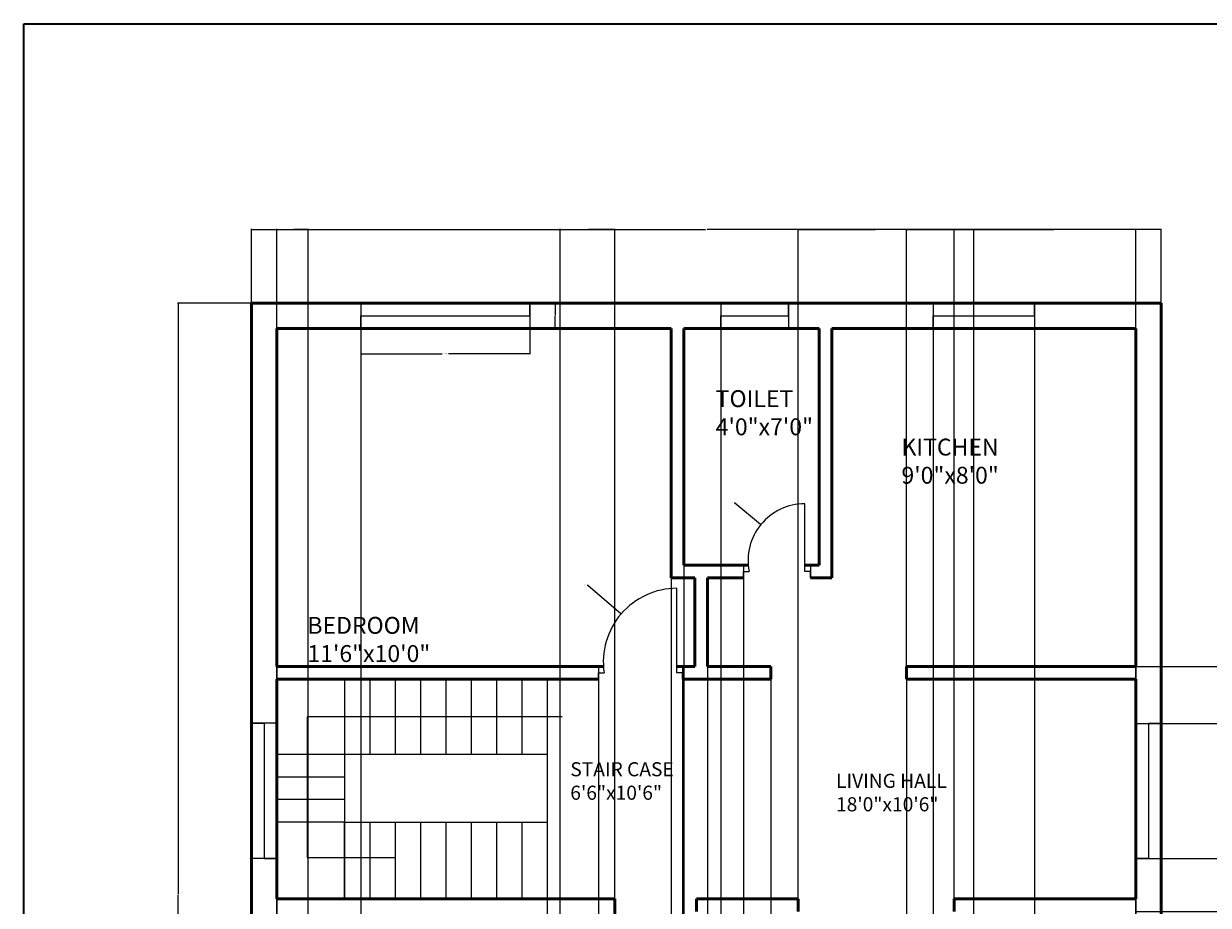
# Model space of a CAD drawing. Units: inches. Extents: x 1860 to 2753, y 1742 to 2419.
# Tile 2 of 4: x 1860 to 2280, y 2106 to 2419. Entities that reach past the tile are written whole.
import ezdxf

# ---------------------------------------------------------------- set-up
doc = ezdxf.new("R2010")
doc.units = ezdxf.units.IN
for name, color, linetype, lineweight in [('A-ANNO-DIMS', 2, 'Continuous', 18), ('A-ANNO-TTLB', 7, 'Continuous', 35), ('A-AREA-IDEN', 7, 'Continuous', 18), ('A-DOOR', 3, 'Continuous', 25), ('A-FLOR-STRS', 7, 'Continuous', 18), ('A-GLAZ', 4, 'Continuous', 18), ('A-WALL', 7, 'Continuous', 50)]:
    doc.layers.add(name, color=color, linetype=linetype, lineweight=lineweight)
doc.styles.get("Standard").update_dxf_attribs({"font": 'arial.ttf'})
doc.dimstyles.get("Standard").update_dxf_attribs({"dimtxt": 0.18, "dimasz": 0.18, "dimexe": 0.18, "dimexo": 0.0625, "dimgap": 0.09, "dimtad": 0, "dimtih": 1, "dimtoh": 1, "dimdec": 4, "dimzin": 0, "dimdsep": 46, "dimtxsty": 'Standard', "dimcen": 0.09, "dimadec": 0, "dimazin": 0, "dimtfac": 1, "dimtdec": 4, "dimtofl": 0, "dimtmove": 0, "dimatfit": 3, "dimfxl": 1, "dimtolj": 1, "dimtzin": 0, "dimarcsym": 0})

# ---------------------------------------------------------------- blocks, each defined once
blk = doc.blocks.new('WIN-24IN')
for p, q in [((0, 9), (0, 0)), ((24, 4.5), (24, 9)), ((24, 9), (24, 0)), ((0, 0), (0, 4.5)), ((0, 4.5), (24, 4.5))]:
    blk.add_line(p, q)
blk = doc.blocks.new('WIN-60IN')
for p, q in [((0, 9), (0, 0)), ((60, 4.5), (60, 9)), ((60, 9), (60, 0)), ((0, 0), (0, 4.5)), ((0, 4.5), (60, 4.5))]:
    blk.add_line(p, q)
blk = doc.blocks.new('*D3')
at = {"layer": 'A-ANNO-DIMS', "color": 0, "lineweight": -2, "transparency": 16777216}
for p, q in [((1979.28, 2311.09), (1979.28, 2301.97)), ((2039.28, 2311.09), (2039.28, 2301.97)), ((1979.46, 2302.15), (2008.16, 2302.15)), ((2039.1, 2302.15), (2010.4, 2302.15))]:
    blk.add_line(p, q, dxfattribs=at)
at = {"layer": 'A-ANNO-DIMS', "color": 0, "transparency": 16777216}
for points in [[(1979.46, 2302.18), (1979.46, 2302.12), (1979.28, 2302.15)], [(2039.1, 2302.18), (2039.1, 2302.12), (2039.28, 2302.15)]]:
    blk.add_solid(points, dxfattribs=at)
at = {"layer": 'Defpoints', "color": 0, "transparency": 16777216}
for p in [(1979.28, 2311.15), (2039.28, 2311.15), (2039.28, 2302.15)]:
    blk.add_point(p, dxfattribs=at)
at = {"layer": 'A-ANNO-DIMS', "color": 0, "transparency": 16777216, "insert": (2009.28, 2302.15), "char_height": 0.18, "attachment_point": 5}
blk.add_mtext('\\A1;WINDOW 60 TYP.', dxfattribs=at)
blk = doc.blocks.new('*D4')
at = {"layer": 'A-ANNO-DIMS', "color": 0, "lineweight": -2, "transparency": 16777216}
for p, q in [((2039.34, 2320.15), (2048.46, 2320.15)), ((2048.28, 2319.97), (2048.28, 2315.83)), ((2048.28, 2311.33), (2048.28, 2315.47)), ((2039.34, 2311.15), (2048.46, 2311.15))]:
    blk.add_line(p, q, dxfattribs=at)
at = {"layer": 'A-ANNO-DIMS', "color": 0, "transparency": 16777216}
for points in [[(2048.25, 2319.97), (2048.31, 2319.97), (2048.28, 2320.15)], [(2048.25, 2311.33), (2048.31, 2311.33), (2048.28, 2311.15)]]:
    blk.add_solid(points, dxfattribs=at)
at = {"layer": 'Defpoints', "color": 0, "transparency": 16777216}
for p in [(2039.28, 2320.15), (2048.28, 2320.15), (2039.28, 2311.15)]:
    blk.add_point(p, dxfattribs=at)
at = {"layer": 'A-ANNO-DIMS', "color": 0, "transparency": 16777216, "insert": (2048.28, 2315.65), "char_height": 0.18, "attachment_point": 5}
blk.add_mtext('\\A1;9 TYP.', dxfattribs=at)
blk = doc.blocks.new('*D7')
at = {"layer": 'A-ANNO-DIMS', "color": 0, "lineweight": -2, "transparency": 16777216}
for p, q in [((1940.47, 2320.21), (1940.47, 2346.43)), ((1940.65, 2346.25), (2101.68, 2346.25)), ((2263.29, 2346.25), (2102.26, 2346.25)), ((2263.47, 2320.21), (2263.47, 2346.43))]:
    blk.add_line(p, q, dxfattribs=at)
at = {"layer": 'A-ANNO-DIMS', "color": 0, "transparency": 16777216}
for points in [[(1940.65, 2346.28), (1940.65, 2346.22), (1940.47, 2346.25)], [(2263.29, 2346.28), (2263.29, 2346.22), (2263.47, 2346.25)]]:
    blk.add_solid(points, dxfattribs=at)
at = {"layer": 'Defpoints', "color": 0, "transparency": 16777216}
for p in [(2263.47, 2346.25), (1940.47, 2320.15), (2263.47, 2320.15)]:
    blk.add_point(p, dxfattribs=at)
at = {"layer": 'A-ANNO-DIMS', "color": 0, "transparency": 16777216, "insert": (2101.97, 2346.25), "char_height": 0.18, "attachment_point": 5}
blk.add_mtext('\\A1;323', dxfattribs=at)
blk = doc.blocks.new('*D8')
at = {"layer": 'A-ANNO-DIMS', "color": 0, "lineweight": -2, "transparency": 16777216}
for p, q in [((1940.41, 2320.15), (1914.19, 2320.15)), ((1914.37, 2319.97), (1914.37, 2110.33)), ((1914.37, 1900.33), (1914.37, 2109.97)), ((1940.41, 1900.15), (1914.19, 1900.15))]:
    blk.add_line(p, q, dxfattribs=at)
at = {"layer": 'A-ANNO-DIMS', "color": 0, "transparency": 16777216}
for points in [[(1914.34, 2319.97), (1914.4, 2319.97), (1914.37, 2320.15)], [(1914.34, 1900.33), (1914.4, 1900.33), (1914.37, 1900.15)]]:
    blk.add_solid(points, dxfattribs=at)
at = {"layer": 'Defpoints', "color": 0, "transparency": 16777216}
for p in [(1914.37, 2320.15), (1940.47, 2320.15), (1940.47, 1900.15)]:
    blk.add_point(p, dxfattribs=at)
at = {"layer": 'A-ANNO-DIMS', "color": 0, "transparency": 16777216, "insert": (1914.37, 2110.15), "char_height": 0.18, "attachment_point": 5}
blk.add_mtext('\\A1;420', dxfattribs=at)
blk = doc.blocks.new('*D9')
at = {"layer": 'A-ANNO-DIMS', "color": 0, "lineweight": -2, "transparency": 16777216}
for p, q in [((1949.47, 2311.09), (1949.47, 1873.87)), ((1979.28, 2311.09), (1979.28, 1873.87)), ((1949.65, 1874.05), (1964, 1874.05)), ((1979.1, 1874.05), (1964.75, 1874.05))]:
    blk.add_line(p, q, dxfattribs=at)
at = {"layer": 'A-ANNO-DIMS', "color": 0, "transparency": 16777216}
for points in [[(1949.65, 1874.08), (1949.65, 1874.02), (1949.47, 1874.05)], [(1979.1, 1874.08), (1979.1, 1874.02), (1979.28, 1874.05)]]:
    blk.add_solid(points, dxfattribs=at)
at = {"layer": 'Defpoints', "color": 0, "transparency": 16777216}
for p in [(1949.47, 2311.15), (1979.28, 2311.15), (1979.28, 1874.05)]:
    blk.add_point(p, dxfattribs=at)
at = {"layer": 'A-ANNO-DIMS', "color": 0, "transparency": 16777216, "insert": (1964.37, 1874.05), "char_height": 0.18, "attachment_point": 5}
blk.add_mtext('\\A1;29.81', dxfattribs=at)
blk = doc.blocks.new('*D10')
at = {"layer": 'A-ANNO-DIMS', "color": 0, "lineweight": -2, "transparency": 16777216}
for p, q in [((2093.97, 2311.09), (2093.97, 1873.87)), ((2107.08, 2311.09), (2107.08, 1873.87)), ((2094.15, 1874.05), (2100.07, 1874.05)), ((2106.9, 1874.05), (2100.98, 1874.05))]:
    blk.add_line(p, q, dxfattribs=at)
at = {"layer": 'A-ANNO-DIMS', "color": 0, "transparency": 16777216}
for points in [[(2094.15, 1874.08), (2094.15, 1874.02), (2093.97, 1874.05)], [(2106.9, 1874.08), (2106.9, 1874.02), (2107.08, 1874.05)]]:
    blk.add_solid(points, dxfattribs=at)
at = {"layer": 'Defpoints', "color": 0, "transparency": 16777216}
for p in [(2093.97, 2311.15), (2107.08, 2311.15), (2107.08, 1874.05)]:
    blk.add_point(p, dxfattribs=at)
at = {"layer": 'A-ANNO-DIMS', "color": 0, "transparency": 16777216, "insert": (2100.52, 1874.05), "char_height": 0.18, "attachment_point": 5}
blk.add_mtext('\\A1;13.107', dxfattribs=at)
blk = doc.blocks.new('*D11')
at = {"layer": 'A-ANNO-DIMS', "color": 0, "lineweight": -2, "transparency": 16777216}
for p, q in [((2182.45, 2311.09), (2182.45, 1873.87)), ((2218.45, 2311.09), (2218.45, 1873.87)), ((2182.63, 1874.05), (2200.24, 1874.05)), ((2218.27, 1874.05), (2200.67, 1874.05))]:
    blk.add_line(p, q, dxfattribs=at)
at = {"layer": 'A-ANNO-DIMS', "color": 0, "transparency": 16777216}
for points in [[(2182.63, 1874.08), (2182.63, 1874.02), (2182.45, 1874.05)], [(2218.27, 1874.08), (2218.27, 1874.02), (2218.45, 1874.05)]]:
    blk.add_solid(points, dxfattribs=at)
at = {"layer": 'Defpoints', "color": 0, "transparency": 16777216}
for p in [(2182.45, 2311.15), (2218.45, 2311.15), (2218.45, 1874.05)]:
    blk.add_point(p, dxfattribs=at)
at = {"layer": 'A-ANNO-DIMS', "color": 0, "transparency": 16777216, "insert": (2200.45, 1874.05), "char_height": 0.18, "attachment_point": 5}
blk.add_mtext('\\A1;36', dxfattribs=at)
blk = doc.blocks.new('*D12')
at = {"layer": 'A-ANNO-DIMS', "color": 0, "lineweight": -2, "transparency": 16777216}
for p, q in [((2218.45, 2311.09), (2218.45, 1873.87)), ((2254.47, 2311.09), (2254.47, 1873.87)), ((2218.63, 1874.05), (2236, 1874.05)), ((2254.29, 1874.05), (2236.93, 1874.05))]:
    blk.add_line(p, q, dxfattribs=at)
at = {"layer": 'A-ANNO-DIMS', "color": 0, "transparency": 16777216}
for points in [[(2218.63, 1874.08), (2218.63, 1874.02), (2218.45, 1874.05)], [(2254.29, 1874.08), (2254.29, 1874.02), (2254.47, 1874.05)]]:
    blk.add_solid(points, dxfattribs=at)
at = {"layer": 'Defpoints', "color": 0, "transparency": 16777216}
for p in [(2218.45, 2311.15), (2254.47, 2311.15), (2254.47, 1874.05)]:
    blk.add_point(p, dxfattribs=at)
at = {"layer": 'A-ANNO-DIMS', "color": 0, "transparency": 16777216, "insert": (2236.46, 1874.05), "char_height": 0.18, "attachment_point": 5}
blk.add_mtext('\\A1;36.016', dxfattribs=at)
blk = doc.blocks.new('*D13')
at = {"layer": 'A-ANNO-DIMS', "color": 0, "lineweight": -2, "transparency": 16777216}
for p, q in [((1949.47, 1909.21), (1949.47, 2346.43)), ((1949.65, 2346.25), (1954.55, 2346.25)), ((1960.35, 2346.25), (1955.46, 2346.25)), ((1960.53, 1909.21), (1960.53, 2346.43))]:
    blk.add_line(p, q, dxfattribs=at)
at = {"layer": 'A-ANNO-DIMS', "color": 0, "transparency": 16777216}
for points in [[(1949.65, 2346.28), (1949.65, 2346.22), (1949.47, 2346.25)], [(1960.35, 2346.28), (1960.35, 2346.22), (1960.53, 2346.25)]]:
    blk.add_solid(points, dxfattribs=at)
at = {"layer": 'Defpoints', "color": 0, "transparency": 16777216}
for p in [(1960.53, 2346.25), (1949.47, 1909.15), (1960.53, 1909.15)]:
    blk.add_point(p, dxfattribs=at)
at = {"layer": 'A-ANNO-DIMS', "color": 0, "transparency": 16777216, "insert": (1955, 2346.25), "char_height": 0.18, "attachment_point": 5}
blk.add_mtext('\\A1;11.063', dxfattribs=at)
blk = doc.blocks.new('*D15')
at = {"layer": 'A-ANNO-DIMS', "color": 0, "lineweight": -2, "transparency": 16777216}
for p, q in [((2050.02, 1909.21), (2050.02, 2346.43)), ((2050.2, 2346.25), (2059.36, 2346.25)), ((2069.29, 2346.25), (2060.13, 2346.25)), ((2069.47, 1920.76), (2069.47, 2346.43))]:
    blk.add_line(p, q, dxfattribs=at)
at = {"layer": 'A-ANNO-DIMS', "color": 0, "transparency": 16777216}
for points in [[(2050.2, 2346.28), (2050.2, 2346.22), (2050.02, 2346.25)], [(2069.29, 2346.28), (2069.29, 2346.22), (2069.47, 2346.25)]]:
    blk.add_solid(points, dxfattribs=at)
at = {"layer": 'Defpoints', "color": 0, "transparency": 16777216}
for p in [(2069.47, 2346.25), (2069.47, 1920.7), (2050.02, 1909.15)]:
    blk.add_point(p, dxfattribs=at)
at = {"layer": 'A-ANNO-DIMS', "color": 0, "transparency": 16777216, "insert": (2059.74, 2346.25), "char_height": 0.18, "attachment_point": 5}
blk.add_mtext('\\A1;19.45', dxfattribs=at)
blk = doc.blocks.new('*D19')
at = {"layer": 'A-ANNO-DIMS', "color": 0, "lineweight": -2, "transparency": 16777216}
for p, q in [((2263.53, 2122.97), (2289.75, 2122.97)), ((2289.57, 2122.79), (2289.57, 2113.74)), ((2289.57, 2104.33), (2289.57, 2113.38)), ((2254.53, 2104.15), (2289.75, 2104.15))]:
    blk.add_line(p, q, dxfattribs=at)
at = {"layer": 'A-ANNO-DIMS', "color": 0, "transparency": 16777216}
for points in [[(2289.54, 2122.79), (2289.6, 2122.79), (2289.57, 2122.97)], [(2289.54, 2104.33), (2289.6, 2104.33), (2289.57, 2104.15)]]:
    blk.add_solid(points, dxfattribs=at)
at = {"layer": 'Defpoints', "color": 0, "transparency": 16777216}
for p in [(2263.47, 2122.97), (2289.57, 2122.97), (2254.47, 2104.15)]:
    blk.add_point(p, dxfattribs=at)
at = {"layer": 'A-ANNO-DIMS', "color": 0, "transparency": 16777216, "insert": (2289.57, 2113.56), "char_height": 0.18, "attachment_point": 5}
blk.add_mtext('\\A1;18.82', dxfattribs=at)
blk = doc.blocks.new('*D20')
at = {"layer": 'A-ANNO-DIMS', "color": 0, "lineweight": -2, "transparency": 16777216}
for p, q in [((2263.53, 2170.97), (2289.75, 2170.97)), ((2289.57, 2170.79), (2289.57, 2147.15)), ((2289.57, 2123.15), (2289.57, 2146.79)), ((2263.53, 2122.97), (2289.75, 2122.97))]:
    blk.add_line(p, q, dxfattribs=at)
at = {"layer": 'A-ANNO-DIMS', "color": 0, "transparency": 16777216}
for points in [[(2289.54, 2170.79), (2289.6, 2170.79), (2289.57, 2170.97)], [(2289.54, 2123.15), (2289.6, 2123.15), (2289.57, 2122.97)]]:
    blk.add_solid(points, dxfattribs=at)
at = {"layer": 'Defpoints', "color": 0, "transparency": 16777216}
for p in [(2263.47, 2170.97), (2289.57, 2170.97), (2263.47, 2122.97)]:
    blk.add_point(p, dxfattribs=at)
at = {"layer": 'A-ANNO-DIMS', "color": 0, "transparency": 16777216, "insert": (2289.57, 2146.97), "char_height": 0.18, "attachment_point": 5}
blk.add_mtext('\\A1;48', dxfattribs=at)
blk = doc.blocks.new('*D21')
at = {"layer": 'A-ANNO-DIMS', "color": 0, "lineweight": -2, "transparency": 16777216}
for p, q in [((2254.53, 2191.15), (2289.75, 2191.15)), ((2289.57, 2190.97), (2289.57, 2181.24)), ((2289.57, 2171.15), (2289.57, 2180.88)), ((2263.53, 2170.97), (2289.75, 2170.97))]:
    blk.add_line(p, q, dxfattribs=at)
at = {"layer": 'A-ANNO-DIMS', "color": 0, "transparency": 16777216}
for points in [[(2289.54, 2190.97), (2289.6, 2190.97), (2289.57, 2191.15)], [(2289.54, 2171.15), (2289.6, 2171.15), (2289.57, 2170.97)]]:
    blk.add_solid(points, dxfattribs=at)
at = {"layer": 'Defpoints', "color": 0, "transparency": 16777216}
for p in [(2254.47, 2191.15), (2289.57, 2191.15), (2263.47, 2170.97)]:
    blk.add_point(p, dxfattribs=at)
at = {"layer": 'A-ANNO-DIMS', "color": 0, "transparency": 16777216, "insert": (2289.57, 2181.06), "char_height": 0.18, "attachment_point": 5}
blk.add_mtext('\\A1;20.18', dxfattribs=at)
blk = doc.blocks.new('*D22')
at = {"layer": 'A-ANNO-DIMS', "color": 0, "lineweight": -2, "transparency": 16777216}
for p, q in [((2196.96, 1972.21), (2196.96, 2346.43)), ((2197.14, 2346.25), (2225.34, 2346.25)), ((2254.29, 2346.25), (2226.09, 2346.25)), ((2254.47, 1972.21), (2254.47, 2346.43))]:
    blk.add_line(p, q, dxfattribs=at)
at = {"layer": 'A-ANNO-DIMS', "color": 0, "transparency": 16777216}
for points in [[(2197.14, 2346.28), (2197.14, 2346.22), (2196.96, 2346.25)], [(2254.29, 2346.28), (2254.29, 2346.22), (2254.47, 2346.25)]]:
    blk.add_solid(points, dxfattribs=at)
at = {"layer": 'Defpoints', "color": 0, "transparency": 16777216}
for p in [(2254.47, 2346.25), (2196.96, 1972.15), (2254.47, 1972.15)]:
    blk.add_point(p, dxfattribs=at)
at = {"layer": 'A-ANNO-DIMS', "color": 0, "transparency": 16777216, "insert": (2225.71, 2346.25), "char_height": 0.18, "attachment_point": 5}
blk.add_mtext('\\A1;57.51', dxfattribs=at)
blk = doc.blocks.new('*D24')
at = {"layer": 'A-ANNO-DIMS', "color": 0, "lineweight": -2, "transparency": 16777216}
for p, q in [((2134.51, 2108.71), (2134.51, 2346.43)), ((2134.69, 2346.25), (2161.84, 2346.25)), ((2189.78, 2346.25), (2162.63, 2346.25)), ((2189.96, 2108.71), (2189.96, 2346.43))]:
    blk.add_line(p, q, dxfattribs=at)
at = {"layer": 'A-ANNO-DIMS', "color": 0, "transparency": 16777216}
for points in [[(2134.69, 2346.28), (2134.69, 2346.22), (2134.51, 2346.25)], [(2189.78, 2346.28), (2189.78, 2346.22), (2189.96, 2346.25)]]:
    blk.add_solid(points, dxfattribs=at)
at = {"layer": 'Defpoints', "color": 0, "transparency": 16777216}
for p in [(2189.96, 2346.25), (2134.51, 2108.65), (2189.96, 2108.65)]:
    blk.add_point(p, dxfattribs=at)
at = {"layer": 'A-ANNO-DIMS', "color": 0, "transparency": 16777216, "insert": (2162.24, 2346.25), "char_height": 0.18, "attachment_point": 5}
blk.add_mtext('\\A1;55.45', dxfattribs=at)
blk = doc.blocks.new('*D25')
at = {"layer": 'A-ANNO-DIMS', "color": 0, "lineweight": -2, "transparency": 16777216}
for p, q in [((2124.88, 2186.59), (2124.88, 1873.87)), ((2172.98, 2186.59), (2172.98, 1873.87)), ((2125.06, 1874.05), (2148.62, 1874.05)), ((2172.8, 1874.05), (2149.24, 1874.05))]:
    blk.add_line(p, q, dxfattribs=at)
at = {"layer": 'A-ANNO-DIMS', "color": 0, "transparency": 16777216}
for points in [[(2125.06, 1874.08), (2125.06, 1874.02), (2124.88, 1874.05)], [(2172.8, 1874.08), (2172.8, 1874.02), (2172.98, 1874.05)]]:
    blk.add_solid(points, dxfattribs=at)
at = {"layer": 'Defpoints', "color": 0, "transparency": 16777216}
for p in [(2124.88, 2186.65), (2172.98, 2186.65), (2172.98, 1874.05)]:
    blk.add_point(p, dxfattribs=at)
at = {"layer": 'A-ANNO-DIMS', "color": 0, "transparency": 16777216, "insert": (2148.93, 1874.05), "char_height": 0.18, "attachment_point": 5}
blk.add_mtext('\\A1;48.1', dxfattribs=at)
blk = doc.blocks.new('*D26')
at = {"layer": 'A-ANNO-DIMS', "color": 0, "lineweight": -2, "transparency": 16777216}
for p, q in [((2172.98, 2191.21), (2172.98, 2346.43)), ((2173.16, 2346.25), (2213.33, 2346.25)), ((2254.29, 2346.25), (2214.12, 2346.25)), ((2254.47, 2191.21), (2254.47, 2346.43))]:
    blk.add_line(p, q, dxfattribs=at)
at = {"layer": 'A-ANNO-DIMS', "color": 0, "transparency": 16777216}
for points in [[(2173.16, 2346.28), (2173.16, 2346.22), (2172.98, 2346.25)], [(2254.29, 2346.28), (2254.29, 2346.22), (2254.47, 2346.25)]]:
    blk.add_solid(points, dxfattribs=at)
at = {"layer": 'Defpoints', "color": 0, "transparency": 16777216}
for p in [(2254.47, 2346.25), (2172.98, 2191.15), (2254.47, 2191.15)]:
    blk.add_point(p, dxfattribs=at)
at = {"layer": 'A-ANNO-DIMS', "color": 0, "transparency": 16777216, "insert": (2213.73, 2346.25), "char_height": 0.18, "attachment_point": 5}
blk.add_mtext('\\A1;81.49', dxfattribs=at)
blk = doc.blocks.new('*D27')
at = {"layer": 'A-ANNO-DIMS', "color": 0, "lineweight": -2, "transparency": 16777216}
for p, q in [((2089.47, 2311.09), (2089.47, 1873.87)), ((2093.97, 2311.09), (2093.97, 1873.87)), ((2089.65, 1874.05), (2091.46, 1874.05)), ((2093.79, 1874.05), (2091.98, 1874.05))]:
    blk.add_line(p, q, dxfattribs=at)
at = {"layer": 'A-ANNO-DIMS', "color": 0, "transparency": 16777216}
for points in [[(2089.65, 1874.08), (2089.65, 1874.02), (2089.47, 1874.05)], [(2093.79, 1874.08), (2093.79, 1874.02), (2093.97, 1874.05)]]:
    blk.add_solid(points, dxfattribs=at)
at = {"layer": 'Defpoints', "color": 0, "transparency": 16777216}
for p in [(2089.47, 2311.15), (2093.97, 2311.15), (2093.97, 1874.05)]:
    blk.add_point(p, dxfattribs=at)
at = {"layer": 'A-ANNO-DIMS', "color": 0, "transparency": 16777216, "insert": (2091.72, 1874.05), "char_height": 0.18, "attachment_point": 5}
blk.add_mtext('\\A1;4.5', dxfattribs=at)
blk = doc.blocks.new('*D28')
at = {"layer": 'A-ANNO-DIMS', "color": 0, "lineweight": -2, "transparency": 16777216}
for p, q in [((2102.3, 2222.59), (2102.3, 1873.87)), ((2115.14, 2222.59), (2115.14, 1873.87)), ((2102.48, 1874.05), (2108.27, 1874.05)), ((2114.96, 1874.05), (2109.18, 1874.05))]:
    blk.add_line(p, q, dxfattribs=at)
at = {"layer": 'A-ANNO-DIMS', "color": 0, "transparency": 16777216}
for points in [[(2102.48, 1874.08), (2102.48, 1874.02), (2102.3, 1874.05)], [(2114.96, 1874.08), (2114.96, 1874.02), (2115.14, 1874.05)]]:
    blk.add_solid(points, dxfattribs=at)
at = {"layer": 'Defpoints', "color": 0, "transparency": 16777216}
for p in [(2102.3, 2222.65), (2115.14, 2222.65), (2115.14, 1874.05)]:
    blk.add_point(p, dxfattribs=at)
at = {"layer": 'A-ANNO-DIMS', "color": 0, "transparency": 16777216, "insert": (2108.72, 1874.05), "char_height": 0.18, "attachment_point": 5}
blk.add_mtext('\\A1;12.834', dxfattribs=at)
blk = doc.blocks.new('*D29')
at = {"layer": 'A-ANNO-DIMS', "color": 0, "lineweight": -2, "transparency": 16777216}
for p, q in [((2102.3, 2191.09), (2102.3, 1873.87)), ((2093.49, 2186.59), (2093.49, 1873.87)), ((2093.67, 1874.05), (2097.51, 1874.05)), ((2102.12, 1874.05), (2098.29, 1874.05))]:
    blk.add_line(p, q, dxfattribs=at)
at = {"layer": 'A-ANNO-DIMS', "color": 0, "transparency": 16777216}
for points in [[(2093.67, 1874.08), (2093.67, 1874.02), (2093.49, 1874.05)], [(2102.12, 1874.08), (2102.12, 1874.02), (2102.3, 1874.05)]]:
    blk.add_solid(points, dxfattribs=at)
at = {"layer": 'Defpoints', "color": 0, "transparency": 16777216}
for p in [(2102.3, 2191.15), (2093.49, 2186.65), (2102.3, 1874.05)]:
    blk.add_point(p, dxfattribs=at)
at = {"layer": 'A-ANNO-DIMS', "color": 0, "transparency": 16777216, "insert": (2097.9, 1874.05), "char_height": 0.18, "attachment_point": 5}
blk.add_mtext('\\A1;8.809', dxfattribs=at)
blk = doc.blocks.new('*D30')
at = {"layer": 'A-ANNO-DIMS', "color": 0, "lineweight": -2, "transparency": 16777216}
for p, q in [((2045.47, 2186.59), (2045.47, 1873.87)), ((2063.65, 2186.59), (2063.65, 1873.87)), ((2045.65, 1874.05), (2054.11, 1874.05)), ((2063.47, 1874.05), (2055.02, 1874.05))]:
    blk.add_line(p, q, dxfattribs=at)
at = {"layer": 'A-ANNO-DIMS', "color": 0, "transparency": 16777216}
for points in [[(2045.65, 1874.08), (2045.65, 1874.02), (2045.47, 1874.05)], [(2063.47, 1874.08), (2063.47, 1874.02), (2063.65, 1874.05)]]:
    blk.add_solid(points, dxfattribs=at)
at = {"layer": 'Defpoints', "color": 0, "transparency": 16777216}
for p in [(2045.47, 2186.65), (2063.65, 2186.65), (2063.65, 1874.05)]:
    blk.add_point(p, dxfattribs=at)
at = {"layer": 'A-ANNO-DIMS', "color": 0, "transparency": 16777216, "insert": (2054.56, 1874.05), "char_height": 0.18, "attachment_point": 5}
blk.add_mtext('\\A1;18.183', dxfattribs=at)
blk = doc.blocks.new('*D53')
at = {"layer": 'A-ANNO-DIMS', "color": 0, "lineweight": -2, "transparency": 16777216}
for p, q in [((2059.64, 2220.05), (2059.82, 2220.05)), ((2059.82, 2220.05), (2071.56, 2209.94)), ((2091.4, 2192.77), (2091.58, 2192.77)), ((2091.49, 2192.68), (2091.49, 2192.86))]:
    blk.add_line(p, q, dxfattribs=at)
at = {"layer": 'A-ANNO-DIMS', "color": 0, "transparency": 16777216}
blk.add_solid([(2071.58, 2209.96), (2071.54, 2209.92), (2071.7, 2209.82)], dxfattribs=at)
at = {"layer": 'Defpoints', "color": 0, "transparency": 16777216}
for p in [(2071.7, 2209.82), (2091.49, 2192.77)]:
    blk.add_point(p, dxfattribs=at)
at = {"layer": 'A-ANNO-DIMS', "color": 0, "transparency": 16777216, "insert": (2059.16, 2220.05), "char_height": 0.18, "attachment_point": 5}
blk.add_mtext('\\A1;R26.13', dxfattribs=at)
blk = doc.blocks.new('*D55')
at = {"layer": 'A-ANNO-DIMS', "color": 0, "lineweight": -2, "transparency": 16777216}
for p, q in [((2111.84, 2249.23), (2112.02, 2249.23)), ((2112.02, 2249.23), (2121.21, 2241.67)), ((2136.79, 2228.77), (2136.97, 2228.77)), ((2136.88, 2228.68), (2136.88, 2228.86))]:
    blk.add_line(p, q, dxfattribs=at)
at = {"layer": 'A-ANNO-DIMS', "color": 0, "transparency": 16777216}
blk.add_solid([(2121.22, 2241.7), (2121.19, 2241.65), (2121.34, 2241.56)], dxfattribs=at)
at = {"layer": 'Defpoints', "color": 0, "transparency": 16777216}
for p in [(2121.34, 2241.56), (2136.88, 2228.77)]:
    blk.add_point(p, dxfattribs=at)
at = {"layer": 'A-ANNO-DIMS', "color": 0, "transparency": 16777216, "insert": (2111.29, 2249.23), "char_height": 0.18, "attachment_point": 5}
blk.add_mtext('\\A1;R20.123', dxfattribs=at)

msp = doc.modelspace()

# ---------------------------------------------------------------- linework, layer by layer
at = {"layer": 'A-ANNO-TTLB'}
msp.add_lwpolyline([(1859.5561, 2419.29), (2753.3204, 2419.29), (2753.3204, 1741.6035), (1859.5561, 1741.6035)], close=True, dxfattribs=at)
at = {"layer": 'A-DOOR'}
for p, q in [((2136.8843, 2224.8976), (2136.8843, 2248.8976)), ((2115.1377, 2227.1476), (2115.1377, 2222.6476)), ((2138.8843, 2227.1476), (2138.8843, 2222.6476)), ((2115.1377, 2222.6476), (2115.1377, 2224.8976)), ((2115.1377, 2224.8976), (2117.1377, 2224.8976)), ((2138.8843, 2224.8976), (2136.8843, 2224.8976)), ((2138.8843, 2222.6476), (2138.8843, 2224.8976)), ((2091.4949, 2188.8976), (2091.4949, 2218.8976)), ((2063.6532, 2191.1476), (2063.6532, 2191.1476)), ((2063.6532, 2191.1476), (2063.6532, 2186.6476)), ((2063.6532, 2186.6476), (2063.6532, 2188.8976)), ((2063.6532, 2188.8976), (2065.6532, 2188.8976)), ((2093.4949, 2188.8976), (2091.4949, 2188.8976)), ((2093.4949, 2191.1476), (2093.4949, 2186.6476)), ((2093.4949, 2186.6476), (2093.4949, 2188.8976))]:
    msp.add_line(p, q, dxfattribs=at)
for centre, radius, end in [((2136.8843, 2228.7741), 20.1235, 191.10666), ((2091.4949, 2192.7677), 26.1299, 188.517535)]:
    msp.add_arc(centre, radius, 90, end, dxfattribs=at)
at = {"layer": 'A-FLOR-STRS'}
for p, q in [((1949.4703, 2186.6476), (1973.4703, 2186.6476)), ((1973.4703, 2186.6476), (1973.4703, 2108.6476)), ((1982.4703, 2186.6476), (1982.4703, 2159.9296)), ((1991.4703, 2186.6476), (1991.4703, 2159.9296)), ((2000.4703, 2186.6476), (2000.4703, 2159.9296)), ((2009.4703, 2186.6476), (2009.4703, 2159.9296)), ((2018.4703, 2186.6476), (2018.4703, 2159.9296)), ((2027.4703, 2186.6476), (2027.4703, 2159.9296)), ((2036.4703, 2186.6476), (2036.4703, 2159.9296)), ((2045.4703, 2186.6476), (2045.4703, 2159.9296)), ((2050.7657, 2173.2886), (1960.21, 2173.2886)), ((1960.21, 2173.2886), (1960.21, 2123.3325)), ((1973.4703, 2159.9296), (1949.4703, 2159.9296)), ((2045.4703, 2159.9296), (1973.4703, 2159.9296)), ((1973.4703, 2151.9296), (1949.4703, 2151.9296)), ((1973.4703, 2143.9296), (1949.4703, 2143.9296)), ((1973.4703, 2135.9296), (1949.4703, 2135.9296)), ((1973.4703, 2108.6476), (1973.4703, 2135.9296)), ((1973.4703, 2135.9296), (2045.4703, 2135.9296)), ((1982.4703, 2135.9296), (1982.4703, 2108.6476)), ((1991.4703, 2135.9296), (1991.4703, 2108.6476)), ((2000.4703, 2135.9296), (2000.4703, 2108.6476)), ((2009.4703, 2135.9296), (2009.4703, 2108.6476)), ((2018.4703, 2135.9296), (2018.4703, 2108.6476)), ((2027.4703, 2135.9296), (2027.4703, 2108.6476)), ((2036.4703, 2135.9296), (2036.4703, 2108.6476)), ((2045.4703, 2135.9296), (2045.4703, 2108.6476)), ((1960.21, 2123.3325), (1991.4703, 2123.3325))]:
    msp.add_line(p, q, dxfattribs=at)
at = {"layer": 'A-GLAZ'}
for p, q in [((2182.4546, 2320.1476), (2182.4546, 2311.1476)), ((2218.4546, 2315.6476), (2218.4546, 2320.1476)), ((2218.4546, 2320.1476), (2218.4546, 2311.1476)), ((2107.0777, 2315.6476), (2107.0777, 2315.6476)), ((2182.4546, 2311.1476), (2182.4546, 2315.6476)), ((2182.4546, 2315.6476), (2218.4546, 2315.6476)), ((2218.4546, 2311.1476), (2218.4546, 2311.1476)), ((1949.4703, 2171.0311), (1940.4703, 2171.0311)), ((1940.4703, 2171.0311), (1944.9703, 2171.0311)), ((1944.9703, 2171.0311), (1944.9703, 2123.0311)), ((2254.4703, 2170.9674), (2263.4703, 2170.9674)), ((2263.4703, 2170.9674), (2258.9703, 2170.9674)), ((2258.9703, 2170.9674), (2258.9703, 2146.9674)), ((2258.9703, 2146.9674), (2258.9703, 2134.9674)), ((2258.9703, 2134.9674), (2258.9703, 2122.9674)), ((1949.4703, 2123.0311), (1940.4703, 2123.0311)), ((1944.9703, 2123.0311), (1949.4703, 2123.0311)), ((2258.9703, 2122.9674), (2254.4703, 2122.9674)), ((2254.4703, 2122.9674), (2263.4703, 2122.9674))]:
    msp.add_line(p, q, dxfattribs=at)
at = {"layer": 'A-WALL'}
for p, q in [((1940.4703, 2320.1476), (2263.4703, 2320.1476)), ((1940.4703, 2320.1476), (2263.4703, 2320.1476)), ((1940.4703, 2320.1476), (1940.4703, 1900.1476)), ((2263.4703, 2320.1476), (2263.4703, 1900.1476)), ((1949.4703, 2311.1476), (2089.4703, 2311.1476)), ((1949.4703, 2311.1476), (1949.4703, 2191.1476)), ((2089.4703, 2311.1476), (2089.4703, 2222.6476)), ((2093.9703, 2311.1476), (2093.9703, 2227.1476)), ((2093.9703, 2311.1476), (2141.9703, 2311.1476)), ((2141.9703, 2311.1476), (2141.9703, 2227.1476)), ((2146.4703, 2311.1476), (2146.4703, 2222.6476)), ((2146.4703, 2311.1476), (2254.4703, 2311.1476)), ((2254.4703, 2311.1476), (2254.4703, 2191.1476)), ((2093.9703, 2227.1476), (2116.8266, 2227.1476)), ((2136.8843, 2227.1476), (2141.9703, 2227.1476)), ((2089.4703, 2222.6476), (2097.804, 2222.6476)), ((2097.804, 2191.1476), (2097.804, 2222.6476)), ((2102.304, 2222.6476), (2102.304, 2191.1476)), ((2102.304, 2222.6476), (2115.1377, 2222.6476)), ((2138.8843, 2222.6476), (2146.4703, 2222.6476)), ((1949.4703, 2191.1476), (2065.4153, 2191.1476)), ((2091.4949, 2191.1476), (2097.804, 2191.1476)), ((2102.304, 2191.1476), (2124.8791, 2191.1476)), ((2124.8791, 2191.1476), (2124.8791, 2186.6476)), ((2172.9826, 2191.1476), (2172.9826, 2186.6476)), ((2172.9826, 2191.1476), (2254.4703, 2191.1476)), ((1949.4703, 2186.6476), (2063.6532, 2186.6476)), ((1949.4703, 2186.6476), (1949.4703, 2108.6476)), ((2093.4949, 2186.6476), (2124.8791, 2186.6476)), ((2172.9826, 2186.6476), (2254.4703, 2186.6476)), ((2254.4703, 2186.6476), (2254.4703, 2108.6476)), ((1949.4703, 2108.6476), (2069.4703, 2108.6476)), ((2069.4703, 2108.6476), (2060.4703, 2108.6476)), ((2069.4703, 1963.1476), (2069.4703, 2108.6476)), ((2098.4703, 2104.1476), (2098.4703, 2108.6476)), ((2098.4703, 2108.6476), (2134.5133, 2108.6476)), ((2134.5133, 2104.1476), (2134.5133, 2108.6476)), ((2189.9627, 2104.1476), (2189.9627, 2108.6476)), ((2189.9627, 2108.6476), (2254.4703, 2108.6476))]:
    msp.add_line(p, q, dxfattribs=at)

# ---------------------------------------------------------------- block references
at = {"layer": 'A-GLAZ'}
for name, p in [('WIN-60IN', (1979.2792, 2311.1476)), ('WIN-24IN', (2107.0777, 2311.1476))]:
    msp.add_blockref(name, p, dxfattribs=at)

# ---------------------------------------------------------------- texts
at = {"layer": 'A-AREA-IDEN', "attachment_point": 1}
for s, width, insert, char_height in [('TOILET\\P4\'0"x7\'0"', 104.54554, (2105.2634, 2289.2226), 6), ('KITCHEN\\P9\'0"x8\'0"', 171.99421, (2171.2214, 2272.0322), 6), ('BEDROOM\\P11\'6"x10\'0"', 110.541734, (1960.2814, 2208.7504), 6), ('STAIR CASE\\P6\'6"x10\'6"', 82.831268, (2053.6381, 2157.1871), 5), ('LIVING HALL\\P18\'0"x10\'6"', 136.305792, (2147.9978, 2153.0819), 5)]:
    msp.add_mtext_dynamic_manual_height_columns(s, width=width, gutter_width=12.5, heights=[0], dxfattribs=dict(at, insert=insert, char_height=char_height))

# ---------------------------------------------------------------- dimensions: what is measured, and where the dimension line sits
at = {"layer": 'A-ANNO-DIMS'}
for base, p1, p2, override, picture, middle in [((2263.4703, 2346.2476), (1940.4703, 2320.1476), (2263.4703, 2320.1476), {"dimdec": 0, "dimlfac": 1, "dimrnd": 0, "dimzin": 0, "dimdsep": 46, "dimlunit": 2}, '*D7', (2101.9703, 2346.2476)), ((1960.5331, 2346.2476), (1949.4703, 1909.1476), (1960.5331, 1909.1476), {"dimdec": 3, "dimlfac": 1, "dimrnd": 0, "dimzin": 0, "dimdsep": 46, "dimlunit": 2}, '*D13', (1955.0017, 2346.2476)), ((2069.4703, 2346.2476), (2050.0189, 1909.1476), (2069.4703, 1920.6989), {"dimdec": 2, "dimlfac": 1, "dimrnd": 0, "dimzin": 0, "dimdsep": 46, "dimlunit": 2}, '*D15', (2059.7446, 2346.2476)), ((2189.9627, 2346.2476), (2134.5133, 2108.6476), (2189.9627, 2108.6476), {"dimdec": 2, "dimlfac": 1, "dimrnd": 0, "dimzin": 0, "dimdsep": 46, "dimlunit": 2}, '*D24', (2162.238, 2346.2476)), ((2254.4703, 2346.2476), (2172.9826, 2191.1476), (2254.4703, 2191.1476), {"dimdec": 2, "dimlfac": 1, "dimrnd": 0, "dimzin": 0, "dimdsep": 46, "dimlunit": 2}, '*D26', (2213.7265, 2346.2476)), ((2254.4703, 2346.2476), (2196.9581, 1972.1476), (2254.4703, 1972.1476), {"dimdec": 2, "dimlfac": 1, "dimrnd": 0, "dimzin": 0, "dimdsep": 46, "dimlunit": 2}, '*D22', (2225.7142, 2346.2476)), ((1979.2792, 1874.0476), (1949.4703, 2311.1476), (1979.2792, 2311.1476), {"dimdec": 2, "dimlfac": 1, "dimrnd": 0, "dimzin": 0, "dimdsep": 46, "dimlunit": 2}, '*D9', (1964.3747, 1874.0476)), ((2093.9703, 1874.0476), (2089.4703, 2311.1476), (2093.9703, 2311.1476), {"dimdec": 1, "dimlfac": 1, "dimrnd": 0, "dimzin": 0, "dimdsep": 46, "dimlunit": 2}, '*D27', (2091.7203, 1874.0476)), ((2107.0777, 1874.0476), (2093.9703, 2311.1476), (2107.0777, 2311.1476), {"dimdec": 3, "dimlfac": 1, "dimrnd": 0, "dimzin": 0, "dimdsep": 46, "dimlunit": 2}, '*D10', (2100.524, 1874.0476)), ((2218.4546, 1874.0476), (2182.4546, 2311.1476), (2218.4546, 2311.1476), {"dimdec": 0, "dimlfac": 1, "dimrnd": 0, "dimzin": 0, "dimdsep": 46, "dimlunit": 2}, '*D11', (2200.4546, 1874.0476)), ((2254.4703, 1874.0476), (2218.4546, 2311.1476), (2254.4703, 2311.1476), {"dimdec": 3, "dimlfac": 1, "dimrnd": 0, "dimzin": 0, "dimdsep": 46, "dimlunit": 2}, '*D12', (2236.4625, 1874.0476)), ((2115.1377, 1874.0476), (2102.304, 2222.6476), (2115.1377, 2222.6476), {"dimdec": 3, "dimlfac": 1, "dimrnd": 0, "dimzin": 0, "dimdsep": 46, "dimlunit": 2}, '*D28', (2108.7208, 1874.0476)), ((2102.304, 1874.0476), (2093.4949, 2186.6476), (2102.304, 2191.1476), {"dimdec": 3, "dimlfac": 1, "dimrnd": 0, "dimzin": 0, "dimdsep": 46, "dimlunit": 2}, '*D29', (2097.8994, 1874.0476)), ((2063.6532, 1874.0476), (2045.4703, 2186.6476), (2063.6532, 2186.6476), {"dimdec": 3, "dimlfac": 1, "dimrnd": 0, "dimzin": 0, "dimdsep": 46, "dimlunit": 2}, '*D30', (2054.5618, 1874.0476)), ((2172.9826, 1874.0476), (2124.8791, 2186.6476), (2172.9826, 2186.6476), {"dimdec": 1, "dimlfac": 1, "dimrnd": 0, "dimzin": 0, "dimdsep": 46, "dimlunit": 2}, '*D25', (2148.9308, 1874.0476))]:
    dim = msp.add_linear_dim(base=base, p1=p1, p2=p2, dimstyle='Standard', override=override, dxfattribs=at)
    dim.commit()
    dim.dimension.update_dxf_attribs({"geometry": picture, "text_midpoint": middle})
for base, p1, p2, override, picture, middle in [((1914.3703, 2320.1476), (1940.4703, 1900.1476), (1940.4703, 2320.1476), {"dimdec": 0, "dimlfac": 1, "dimrnd": 0, "dimzin": 0, "dimdsep": 46, "dimlunit": 2}, '*D8', (1914.3703, 2110.1476)), ((2289.5703, 2191.1476), (2263.4703, 2170.9674), (2254.4703, 2191.1476), {"dimdec": 2, "dimlfac": 1, "dimrnd": 0, "dimzin": 0, "dimdsep": 46, "dimlunit": 2}, '*D21', (2289.5703, 2181.0575)), ((2289.5703, 2170.9674), (2263.4703, 2122.9674), (2263.4703, 2170.9674), {"dimdec": 0, "dimlfac": 1, "dimrnd": 0, "dimzin": 0, "dimdsep": 46, "dimlunit": 2}, '*D20', (2289.5703, 2146.9674)), ((2289.5703, 2122.9674), (2254.4703, 2104.1476), (2263.4703, 2122.9674), {"dimdec": 2, "dimlfac": 1, "dimrnd": 0, "dimzin": 0, "dimdsep": 46, "dimlunit": 2}, '*D19', (2289.5703, 2113.5575))]:
    dim = msp.add_linear_dim(base=base, p1=p1, p2=p2, angle=90, dimstyle='Standard', override=override, dxfattribs=at)
    dim.commit()
    dim.dimension.update_dxf_attribs({"geometry": picture, "text_midpoint": middle})
dim = msp.add_linear_dim(base=(2048.2792, 2320.1476), p1=(2039.2792, 2311.1476), p2=(2039.2792, 2320.1476), angle=90, text='<> TYP.', dimstyle='Standard', override={"dimdec": 0, "dimlfac": 1, "dimrnd": 0, "dimzin": 0, "dimdsep": 46, "dimlunit": 2}, dxfattribs=at)
dim.commit()
dim.dimension.update_dxf_attribs({"geometry": '*D4', "text_midpoint": (2048.2792, 2315.6476)})
dim = msp.add_linear_dim(base=(2039.2792, 2302.1476), p1=(1979.2792, 2311.1476), p2=(2039.2792, 2311.1476), text='WINDOW <> TYP.', dimstyle='Standard', override={"dimdec": 0, "dimlfac": 1, "dimrnd": 0, "dimzin": 0, "dimdsep": 46, "dimlunit": 2}, dxfattribs=at)
dim.commit()
dim.dimension.update_dxf_attribs({"geometry": '*D3', "text_midpoint": (2009.2792, 2302.1476)})
for center, mpoint, override, picture, middle in [((2136.8843, 2228.7741), (2121.3449, 2241.5601), {"dimdec": 3, "dimlfac": 1, "dimrnd": 0, "dimzin": 0, "dimdsep": 46, "dimlunit": 2}, '*D55', (2111.2915, 2249.2317)), ((2091.4949, 2192.7677), (2071.697, 2209.821), {"dimdec": 2, "dimlfac": 1, "dimrnd": 0, "dimzin": 0, "dimdsep": 46, "dimlunit": 2}, '*D53', (2059.1584, 2220.0529))]:
    dim = msp.add_radius_dim(center=center, mpoint=mpoint, dimstyle='Standard', override=override, dxfattribs=at)
    dim.commit()
    dim.dimension.update_dxf_attribs({"geometry": picture, "text_midpoint": middle, "dimtype": 164})

doc.saveas('drawing.dxf')
